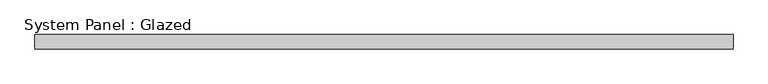
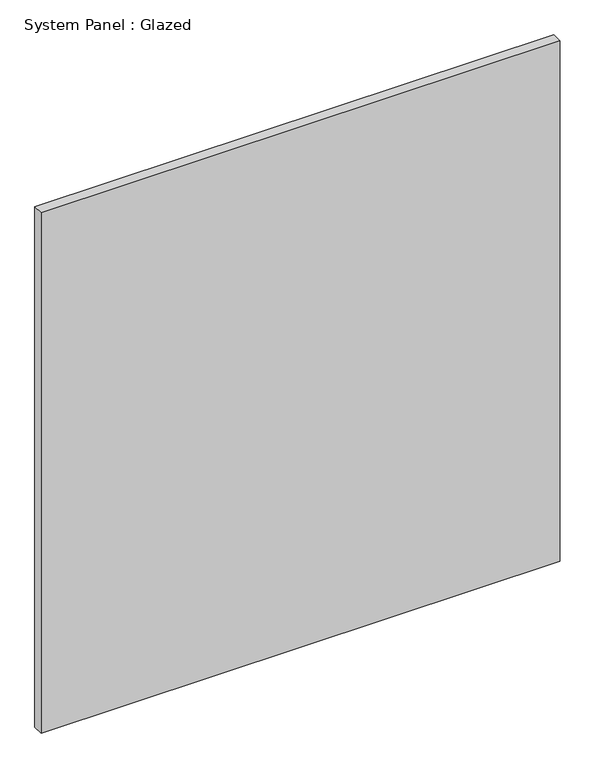
"""IFC4 building model written with IfcOpenShell, lengths in millimetres: plate geometry, System Panel : Glazed."""

from ifc_helpers import new_model, si_unit, origin, origin_with_axes, place, context, project, spatial, polyline, outline, extrude, source, transform, mapped, element, save


def system_panel_glazed_a6784857(model_context):
    return source(origin(), model_context, "Body", "SweptSolid", [
        extrude(outline(polyline([(622.3, 19.05), (-622.3, 19.05), (-622.3, 44.45), (622.3, 44.45), (622.3, 19.05)])), origin_with_axes(), (0.0, 0.0, 1.0), 1317.9920522),
    ])


if __name__ == "__main__":
    model = new_model("IFC4")
    model_context = context("Model", 3, world=origin())
    ifc_project = project(units=[si_unit("LENGTHUNIT", "METRE", prefix="MILLI")], contexts=[model_context])
    site = spatial("IfcSite", under=ifc_project)
    building = spatial("IfcBuilding", under=site)
    placement = place(None, origin())
    system_panel_glazed_shape = system_panel_glazed_a6784857(model_context)
    element("IfcPlate", 1, ObjectType="System Panel : Glazed", at=placement, inside=building, context=model_context, shape_type="MappedRepresentation", body=[
        mapped(system_panel_glazed_shape, transform((0.0, 0.0, 0.0), x_axis=(1.0, 0.0, 0.0), y_axis=(0.0, 1.0, 0.0), z_axis=(0.0, 0.0, 1.0))),
    ])
    save(model, "model.ifc")

# Revit data of these elements
# Type "System Panel : Glazed"
#   Construction Type Id = "GSP4R"
#   Analytic Construction = "1/8 in Pilkington single glazing"
#   Visual Light Transmittance = 0.9
#   Solar Heat Gain Coefficient = 0.86
#   Heat Transfer Coefficient (U) = 1.18115 BTU/(h·ft²·°F)
#   Define Thermal Properties by = 1
# Element 1 (IfcPlate, "System Panel : Glazed")
#   Materials on its faces: "Glass"
# Materials
#   "Glass": class "Glass", colour RGB 0 128 192, transparency 0.75, Description = "Soda Lime Glass", Cost = 0
